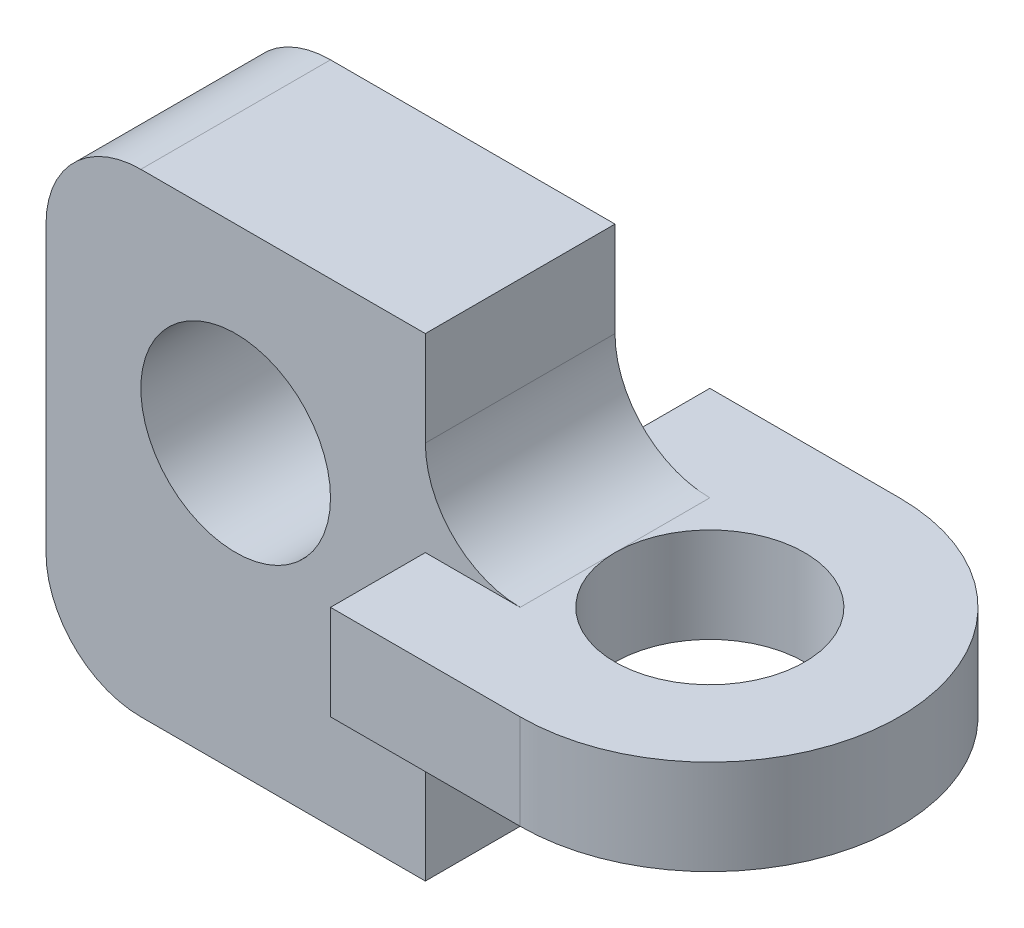
ISO-10303-21;
HEADER;
FILE_DESCRIPTION(('STEP AP214'),'2;1');
FILE_NAME('part.step','',(''),(''),'','','');
FILE_SCHEMA(('AUTOMOTIVE_DESIGN { 1 0 10303 214 1 1 1 1 }'));
ENDSEC;
DATA;
#1=APPLICATION_CONTEXT('core data for automotive mechanical design processes');
#2=APPLICATION_PROTOCOL_DEFINITION('international standard','automotive_design',2000,#1);
#3=PRODUCT_CONTEXT('',#1,'mechanical');
#4=PRODUCT('Part','Part','',(#3));
#5=PRODUCT_RELATED_PRODUCT_CATEGORY('part','',(#4));
#6=PRODUCT_DEFINITION_FORMATION('','',#4);
#7=PRODUCT_DEFINITION_CONTEXT('part definition',#1,'design');
#8=PRODUCT_DEFINITION('design','',#6,#7);
#9=PRODUCT_DEFINITION_SHAPE('','',#8);
#10=(LENGTH_UNIT() NAMED_UNIT(*) SI_UNIT(.MILLI.,.METRE.));
#11=(NAMED_UNIT(*) PLANE_ANGLE_UNIT() SI_UNIT($,.RADIAN.));
#12=(NAMED_UNIT(*) SI_UNIT($,.STERADIAN.) SOLID_ANGLE_UNIT());
#13=UNCERTAINTY_MEASURE_WITH_UNIT(LENGTH_MEASURE(1.E-05),#10,'distance_accuracy_value','');
#14=(GEOMETRIC_REPRESENTATION_CONTEXT(3) GLOBAL_UNCERTAINTY_ASSIGNED_CONTEXT((#13)) GLOBAL_UNIT_ASSIGNED_CONTEXT((#10,
#11,#12)) REPRESENTATION_CONTEXT('',''));
#15=CARTESIAN_POINT('',(0.,0.,0.));
#16=DIRECTION('',(0.,0.,1.));
#17=DIRECTION('',(1.,0.,0.));
#18=AXIS2_PLACEMENT_3D('',#15,#16,#17);
#19=CARTESIAN_POINT('',(40.,-5.,0.));
#20=DIRECTION('',(0.,-1.,0.));
#21=DIRECTION('',(0.,0.,-1.));
#22=AXIS2_PLACEMENT_3D('',#19,#20,#21);
#23=CYLINDRICAL_SURFACE('',#22,20.);
#24=DIRECTION('',(0.,-1.,0.));
#25=VECTOR('',#24,1.);
#26=CARTESIAN_POINT('',(40.,5.,20.));
#27=LINE('',#26,#25);
#28=CARTESIAN_POINT('',(40.,-5.,20.));
#29=VERTEX_POINT('',#28);
#30=CARTESIAN_POINT('',(40.,5.,20.));
#31=VERTEX_POINT('',#30);
#32=EDGE_CURVE('E178',#29,#31,#27,.F.);
#33=ORIENTED_EDGE('',*,*,#32,.F.);
#34=CARTESIAN_POINT('',(40.,-5.,0.));
#35=DIRECTION('',(0.,1.,0.));
#36=DIRECTION('',(0.,0.,1.));
#37=AXIS2_PLACEMENT_3D('',#34,#35,#36);
#38=CIRCLE('',#37,20.);
#39=CARTESIAN_POINT('',(40.,-5.,-20.));
#40=VERTEX_POINT('',#39);
#41=EDGE_CURVE('E245',#40,#29,#38,.F.);
#42=ORIENTED_EDGE('',*,*,#41,.F.);
#43=DIRECTION('',(0.,-1.,0.));
#44=VECTOR('',#43,1.);
#45=CARTESIAN_POINT('',(40.,5.,-20.));
#46=LINE('',#45,#44);
#47=CARTESIAN_POINT('',(40.,5.,-20.));
#48=VERTEX_POINT('',#47);
#49=EDGE_CURVE('E243',#48,#40,#46,.T.);
#50=ORIENTED_EDGE('',*,*,#49,.F.);
#51=CARTESIAN_POINT('',(40.,5.,0.));
#52=DIRECTION('',(0.,1.,0.));
#53=DIRECTION('',(0.,0.,1.));
#54=AXIS2_PLACEMENT_3D('',#51,#52,#53);
#55=CIRCLE('',#54,20.);
#56=EDGE_CURVE('E249',#31,#48,#55,.T.);
#57=ORIENTED_EDGE('',*,*,#56,.F.);
#58=EDGE_LOOP('',(#33,#42,#50,#57));
#59=FACE_BOUND('',#58,.T.);
#60=ADVANCED_FACE('F41',(#59),#23,.T.);
#61=CARTESIAN_POINT('',(20.,-25.,10.));
#62=DIRECTION('',(-1.,0.,0.));
#63=DIRECTION('',(0.,0.,1.));
#64=AXIS2_PLACEMENT_3D('',#61,#62,#63);
#65=PLANE('',#64);
#66=DIRECTION('',(0.,1.,0.));
#67=VECTOR('',#66,1.);
#68=CARTESIAN_POINT('',(20.,-25.,10.));
#69=LINE('',#68,#67);
#70=CARTESIAN_POINT('',(20.,15.,10.));
#71=VERTEX_POINT('',#70);
#72=CARTESIAN_POINT('',(20.,25.,10.));
#73=VERTEX_POINT('',#72);
#74=EDGE_CURVE('E203',#71,#73,#69,.T.);
#75=ORIENTED_EDGE('',*,*,#74,.F.);
#76=DIRECTION('',(0.,0.,1.));
#77=VECTOR('',#76,1.);
#78=CARTESIAN_POINT('',(20.,15.,10.));
#79=LINE('',#78,#77);
#80=CARTESIAN_POINT('',(20.,15.,-10.));
#81=VERTEX_POINT('',#80);
#82=EDGE_CURVE('E270',#71,#81,#79,.F.);
#83=ORIENTED_EDGE('',*,*,#82,.T.);
#84=DIRECTION('',(0.,1.,0.));
#85=VECTOR('',#84,1.);
#86=CARTESIAN_POINT('',(20.,-25.,-10.));
#87=LINE('',#86,#85);
#88=CARTESIAN_POINT('',(20.,25.,-10.));
#89=VERTEX_POINT('',#88);
#90=EDGE_CURVE('E188',#81,#89,#87,.T.);
#91=ORIENTED_EDGE('',*,*,#90,.T.);
#92=DIRECTION('',(0.,0.,-1.));
#93=VECTOR('',#92,1.);
#94=CARTESIAN_POINT('',(20.,25.,10.));
#95=LINE('',#94,#93);
#96=EDGE_CURVE('E240',#73,#89,#95,.T.);
#97=ORIENTED_EDGE('',*,*,#96,.F.);
#98=EDGE_LOOP('',(#75,#83,#91,#97));
#99=FACE_BOUND('',#98,.T.);
#100=ADVANCED_FACE('F282',(#99),#65,.F.);
#101=CARTESIAN_POINT('',(20.,-25.,-10.));
#102=VERTEX_POINT('',#101);
#103=CARTESIAN_POINT('',(20.,-15.,-10.));
#104=VERTEX_POINT('',#103);
#105=EDGE_CURVE('E194',#102,#104,#87,.T.);
#106=ORIENTED_EDGE('',*,*,#105,.T.);
#107=DIRECTION('',(0.,0.,1.));
#108=VECTOR('',#107,1.);
#109=CARTESIAN_POINT('',(20.,-15.,10.));
#110=LINE('',#109,#108);
#111=CARTESIAN_POINT('',(20.,-15.,10.));
#112=VERTEX_POINT('',#111);
#113=EDGE_CURVE('E250',#104,#112,#110,.T.);
#114=ORIENTED_EDGE('',*,*,#113,.T.);
#115=CARTESIAN_POINT('',(20.,-25.,10.));
#116=VERTEX_POINT('',#115);
#117=EDGE_CURVE('E198',#116,#112,#69,.T.);
#118=ORIENTED_EDGE('',*,*,#117,.F.);
#119=DIRECTION('',(0.,0.,-1.));
#120=VECTOR('',#119,1.);
#121=CARTESIAN_POINT('',(20.,-25.,10.));
#122=LINE('',#121,#120);
#123=EDGE_CURVE('E209',#116,#102,#122,.T.);
#124=ORIENTED_EDGE('',*,*,#123,.T.);
#125=EDGE_LOOP('',(#106,#114,#118,#124));
#126=FACE_BOUND('',#125,.T.);
#127=ADVANCED_FACE('F315',(#126),#65,.F.);
#128=CARTESIAN_POINT('',(20.,25.,10.));
#129=DIRECTION('',(0.,-1.,0.));
#130=DIRECTION('',(0.,0.,-1.));
#131=AXIS2_PLACEMENT_3D('',#128,#129,#130);
#132=PLANE('',#131);
#133=DIRECTION('',(-1.,0.,0.));
#134=VECTOR('',#133,1.);
#135=CARTESIAN_POINT('',(20.,25.,-10.));
#136=LINE('',#135,#134);
#137=CARTESIAN_POINT('',(-9.99999999999992,25.,-10.));
#138=VERTEX_POINT('',#137);
#139=EDGE_CURVE('E213',#89,#138,#136,.T.);
#140=ORIENTED_EDGE('',*,*,#139,.T.);
#141=DIRECTION('',(0.,0.,-1.));
#142=VECTOR('',#141,1.);
#143=CARTESIAN_POINT('',(-9.99999999999992,25.,10.));
#144=LINE('',#143,#142);
#145=CARTESIAN_POINT('',(-9.99999999999992,25.,10.));
#146=VERTEX_POINT('',#145);
#147=EDGE_CURVE('E233',#146,#138,#144,.T.);
#148=ORIENTED_EDGE('',*,*,#147,.F.);
#149=DIRECTION('',(-1.,0.,0.));
#150=VECTOR('',#149,1.);
#151=CARTESIAN_POINT('',(20.,25.,10.));
#152=LINE('',#151,#150);
#153=EDGE_CURVE('E200',#73,#146,#152,.T.);
#154=ORIENTED_EDGE('',*,*,#153,.F.);
#155=ORIENTED_EDGE('',*,*,#96,.T.);
#156=EDGE_LOOP('',(#140,#148,#154,#155));
#157=FACE_BOUND('',#156,.T.);
#158=ADVANCED_FACE('F333',(#157),#132,.F.);
#159=CARTESIAN_POINT('',(-10.,15.,10.));
#160=DIRECTION('',(0.,0.,-1.));
#161=DIRECTION('',(-1.,0.,0.));
#162=AXIS2_PLACEMENT_3D('',#159,#160,#161);
#163=CYLINDRICAL_SURFACE('',#162,10.);
#164=CARTESIAN_POINT('',(-10.,15.,-10.));
#165=DIRECTION('',(0.,0.,1.));
#166=DIRECTION('',(1.,0.,0.));
#167=AXIS2_PLACEMENT_3D('',#164,#165,#166);
#168=CIRCLE('',#167,10.);
#169=CARTESIAN_POINT('',(-20.,14.9999999999999,-10.));
#170=VERTEX_POINT('',#169);
#171=EDGE_CURVE('E214',#138,#170,#168,.T.);
#172=ORIENTED_EDGE('',*,*,#171,.T.);
#173=DIRECTION('',(0.,0.,-1.));
#174=VECTOR('',#173,1.);
#175=CARTESIAN_POINT('',(-20.,14.9999999999999,10.));
#176=LINE('',#175,#174);
#177=CARTESIAN_POINT('',(-20.,14.9999999999999,10.));
#178=VERTEX_POINT('',#177);
#179=EDGE_CURVE('E234',#178,#170,#176,.T.);
#180=ORIENTED_EDGE('',*,*,#179,.F.);
#181=CARTESIAN_POINT('',(-10.,15.,10.));
#182=DIRECTION('',(0.,0.,1.));
#183=DIRECTION('',(1.,0.,0.));
#184=AXIS2_PLACEMENT_3D('',#181,#182,#183);
#185=CIRCLE('',#184,10.);
#186=EDGE_CURVE('E201',#146,#178,#185,.T.);
#187=ORIENTED_EDGE('',*,*,#186,.F.);
#188=ORIENTED_EDGE('',*,*,#147,.T.);
#189=EDGE_LOOP('',(#172,#180,#187,#188));
#190=FACE_BOUND('',#189,.T.);
#191=ADVANCED_FACE('F335',(#190),#163,.T.);
#192=CARTESIAN_POINT('',(-20.,-14.9999999999999,10.));
#193=DIRECTION('',(1.,0.,0.));
#194=DIRECTION('',(0.,0.,-1.));
#195=AXIS2_PLACEMENT_3D('',#192,#193,#194);
#196=PLANE('',#195);
#197=DIRECTION('',(0.,-1.,0.));
#198=VECTOR('',#197,1.);
#199=CARTESIAN_POINT('',(-20.,-14.9999999999999,-10.));
#200=LINE('',#199,#198);
#201=CARTESIAN_POINT('',(-20.,-15.,-10.));
#202=VERTEX_POINT('',#201);
#203=EDGE_CURVE('E220',#170,#202,#200,.T.);
#204=ORIENTED_EDGE('',*,*,#203,.T.);
#205=DIRECTION('',(0.,0.,-1.));
#206=VECTOR('',#205,1.);
#207=CARTESIAN_POINT('',(-20.,-15.,10.));
#208=LINE('',#207,#206);
#209=CARTESIAN_POINT('',(-20.,-15.,10.));
#210=VERTEX_POINT('',#209);
#211=EDGE_CURVE('E227',#210,#202,#208,.T.);
#212=ORIENTED_EDGE('',*,*,#211,.F.);
#213=DIRECTION('',(0.,-1.,0.));
#214=VECTOR('',#213,1.);
#215=CARTESIAN_POINT('',(-20.,-14.9999999999999,10.));
#216=LINE('',#215,#214);
#217=EDGE_CURVE('E202',#178,#210,#216,.T.);
#218=ORIENTED_EDGE('',*,*,#217,.F.);
#219=ORIENTED_EDGE('',*,*,#179,.T.);
#220=EDGE_LOOP('',(#204,#212,#218,#219));
#221=FACE_BOUND('',#220,.T.);
#222=ADVANCED_FACE('F327',(#221),#196,.F.);
#223=CARTESIAN_POINT('',(-10.,-15.,10.));
#224=DIRECTION('',(0.,0.,-1.));
#225=DIRECTION('',(-1.,0.,0.));
#226=AXIS2_PLACEMENT_3D('',#223,#224,#225);
#227=CYLINDRICAL_SURFACE('',#226,10.);
#228=CARTESIAN_POINT('',(-10.,-15.,-10.));
#229=DIRECTION('',(0.,0.,1.));
#230=DIRECTION('',(-1.,0.,0.));
#231=AXIS2_PLACEMENT_3D('',#228,#229,#230);
#232=CIRCLE('',#231,10.);
#233=CARTESIAN_POINT('',(-9.99999999999993,-25.,-10.));
#234=VERTEX_POINT('',#233);
#235=EDGE_CURVE('E218',#202,#234,#232,.T.);
#236=ORIENTED_EDGE('',*,*,#235,.T.);
#237=DIRECTION('',(0.,0.,-1.));
#238=VECTOR('',#237,1.);
#239=CARTESIAN_POINT('',(-9.99999999999993,-25.,10.));
#240=LINE('',#239,#238);
#241=CARTESIAN_POINT('',(-9.99999999999993,-25.,10.));
#242=VERTEX_POINT('',#241);
#243=EDGE_CURVE('E223',#242,#234,#240,.T.);
#244=ORIENTED_EDGE('',*,*,#243,.F.);
#245=CARTESIAN_POINT('',(-10.,-15.,10.));
#246=DIRECTION('',(0.,0.,1.));
#247=DIRECTION('',(-1.,0.,0.));
#248=AXIS2_PLACEMENT_3D('',#245,#246,#247);
#249=CIRCLE('',#248,10.);
#250=EDGE_CURVE('E210',#210,#242,#249,.T.);
#251=ORIENTED_EDGE('',*,*,#250,.F.);
#252=ORIENTED_EDGE('',*,*,#211,.T.);
#253=EDGE_LOOP('',(#236,#244,#251,#252));
#254=FACE_BOUND('',#253,.T.);
#255=ADVANCED_FACE('F322',(#254),#227,.T.);
#256=CARTESIAN_POINT('',(20.,-25.,10.));
#257=DIRECTION('',(0.,1.,0.));
#258=DIRECTION('',(-1.,0.,0.));
#259=AXIS2_PLACEMENT_3D('',#256,#257,#258);
#260=PLANE('',#259);
#261=DIRECTION('',(1.,0.,0.));
#262=VECTOR('',#261,1.);
#263=CARTESIAN_POINT('',(20.,-25.,-10.));
#264=LINE('',#263,#262);
#265=EDGE_CURVE('E222',#234,#102,#264,.T.);
#266=ORIENTED_EDGE('',*,*,#265,.T.);
#267=ORIENTED_EDGE('',*,*,#123,.F.);
#268=DIRECTION('',(1.,0.,0.));
#269=VECTOR('',#268,1.);
#270=CARTESIAN_POINT('',(20.,-25.,10.));
#271=LINE('',#270,#269);
#272=EDGE_CURVE('E207',#242,#116,#271,.T.);
#273=ORIENTED_EDGE('',*,*,#272,.F.);
#274=ORIENTED_EDGE('',*,*,#243,.T.);
#275=EDGE_LOOP('',(#266,#267,#273,#274));
#276=FACE_BOUND('',#275,.T.);
#277=ADVANCED_FACE('F318',(#276),#260,.F.);
#278=CARTESIAN_POINT('',(-10.,15.,10.));
#279=DIRECTION('',(0.,0.,1.));
#280=DIRECTION('',(1.,0.,0.));
#281=AXIS2_PLACEMENT_3D('',#278,#279,#280);
#282=PLANE('',#281);
#283=CARTESIAN_POINT('',(0.,5.00000000000001,10.));
#284=DIRECTION('',(0.,0.,1.));
#285=DIRECTION('',(1.,0.,0.));
#286=AXIS2_PLACEMENT_3D('',#283,#284,#285);
#287=CIRCLE('',#286,10.);
#288=CARTESIAN_POINT('',(10.,5.00000000000001,10.));
#289=VERTEX_POINT('',#288);
#290=EDGE_CURVE('E501',#289,#289,#287,.T.);
#291=ORIENTED_EDGE('',*,*,#290,.F.);
#292=EDGE_LOOP('',(#291));
#293=FACE_BOUND('',#292,.T.);
#294=ORIENTED_EDGE('',*,*,#117,.T.);
#295=CARTESIAN_POINT('',(30.,-15.,10.));
#296=DIRECTION('',(0.,0.,1.));
#297=DIRECTION('',(1.,0.,0.));
#298=AXIS2_PLACEMENT_3D('',#295,#296,#297);
#299=CIRCLE('',#298,10.);
#300=CARTESIAN_POINT('',(30.,-5.,10.));
#301=VERTEX_POINT('',#300);
#302=EDGE_CURVE('E267',#112,#301,#299,.F.);
#303=ORIENTED_EDGE('',*,*,#302,.T.);
#304=DIRECTION('',(1.,0.,0.));
#305=VECTOR('',#304,1.);
#306=CARTESIAN_POINT('',(0.,-5.,10.));
#307=LINE('',#306,#305);
#308=CARTESIAN_POINT('',(20.,-5.,10.));
#309=VERTEX_POINT('',#308);
#310=EDGE_CURVE('E260',#309,#301,#307,.T.);
#311=ORIENTED_EDGE('',*,*,#310,.F.);
#312=CARTESIAN_POINT('',(20.,5.,10.));
#313=VERTEX_POINT('',#312);
#314=EDGE_CURVE('E199',#309,#313,#69,.T.);
#315=ORIENTED_EDGE('',*,*,#314,.T.);
#316=DIRECTION('',(-1.,0.,0.));
#317=VECTOR('',#316,1.);
#318=CARTESIAN_POINT('',(-10.,5.,10.));
#319=LINE('',#318,#317);
#320=CARTESIAN_POINT('',(30.,5.,10.));
#321=VERTEX_POINT('',#320);
#322=EDGE_CURVE('E163',#321,#313,#319,.T.);
#323=ORIENTED_EDGE('',*,*,#322,.F.);
#324=CARTESIAN_POINT('',(30.,15.,10.));
#325=DIRECTION('',(0.,0.,1.));
#326=DIRECTION('',(1.,0.,0.));
#327=AXIS2_PLACEMENT_3D('',#324,#325,#326);
#328=CIRCLE('',#327,10.);
#329=EDGE_CURVE('E49',#321,#71,#328,.F.);
#330=ORIENTED_EDGE('',*,*,#329,.T.);
#331=ORIENTED_EDGE('',*,*,#74,.T.);
#332=ORIENTED_EDGE('',*,*,#153,.T.);
#333=ORIENTED_EDGE('',*,*,#186,.T.);
#334=ORIENTED_EDGE('',*,*,#217,.T.);
#335=ORIENTED_EDGE('',*,*,#250,.T.);
#336=ORIENTED_EDGE('',*,*,#272,.T.);
#337=EDGE_LOOP('',(#294,#303,#311,#315,#323,#330,#331,#332,#333,#334,#335,#336));
#338=FACE_BOUND('',#337,.T.);
#339=ADVANCED_FACE('F277',(#293,#338),#282,.T.);
#340=CARTESIAN_POINT('',(-10.,15.,-10.));
#341=DIRECTION('',(0.,0.,1.));
#342=DIRECTION('',(1.,0.,0.));
#343=AXIS2_PLACEMENT_3D('',#340,#341,#342);
#344=PLANE('',#343);
#345=CARTESIAN_POINT('',(0.,5.00000000000001,-10.));
#346=DIRECTION('',(0.,0.,1.));
#347=DIRECTION('',(1.,0.,0.));
#348=AXIS2_PLACEMENT_3D('',#345,#346,#347);
#349=CIRCLE('',#348,10.);
#350=CARTESIAN_POINT('',(10.,5.00000000000001,-10.));
#351=VERTEX_POINT('',#350);
#352=EDGE_CURVE('E44',#351,#351,#349,.T.);
#353=ORIENTED_EDGE('',*,*,#352,.T.);
#354=EDGE_LOOP('',(#353));
#355=FACE_BOUND('',#354,.T.);
#356=ORIENTED_EDGE('',*,*,#105,.F.);
#357=ORIENTED_EDGE('',*,*,#265,.F.);
#358=ORIENTED_EDGE('',*,*,#235,.F.);
#359=ORIENTED_EDGE('',*,*,#203,.F.);
#360=ORIENTED_EDGE('',*,*,#171,.F.);
#361=ORIENTED_EDGE('',*,*,#139,.F.);
#362=ORIENTED_EDGE('',*,*,#90,.F.);
#363=CARTESIAN_POINT('',(30.,15.,-10.));
#364=DIRECTION('',(0.,0.,1.));
#365=DIRECTION('',(1.,0.,0.));
#366=AXIS2_PLACEMENT_3D('',#363,#364,#365);
#367=CIRCLE('',#366,10.);
#368=CARTESIAN_POINT('',(30.,5.,-10.));
#369=VERTEX_POINT('',#368);
#370=EDGE_CURVE('E11',#81,#369,#367,.T.);
#371=ORIENTED_EDGE('',*,*,#370,.T.);
#372=DIRECTION('',(1.,0.,0.));
#373=VECTOR('',#372,1.);
#374=CARTESIAN_POINT('',(0.,5.,-10.));
#375=LINE('',#374,#373);
#376=CARTESIAN_POINT('',(20.,5.,-10.));
#377=VERTEX_POINT('',#376);
#378=EDGE_CURVE('E257',#377,#369,#375,.T.);
#379=ORIENTED_EDGE('',*,*,#378,.F.);
#380=CARTESIAN_POINT('',(20.,-5.,-10.));
#381=VERTEX_POINT('',#380);
#382=EDGE_CURVE('E190',#381,#377,#87,.T.);
#383=ORIENTED_EDGE('',*,*,#382,.F.);
#384=DIRECTION('',(-1.,0.,0.));
#385=VECTOR('',#384,1.);
#386=CARTESIAN_POINT('',(-10.,-5.,-10.));
#387=LINE('',#386,#385);
#388=CARTESIAN_POINT('',(30.,-5.,-10.));
#389=VERTEX_POINT('',#388);
#390=EDGE_CURVE('E253',#389,#381,#387,.T.);
#391=ORIENTED_EDGE('',*,*,#390,.F.);
#392=CARTESIAN_POINT('',(30.,-15.,-10.));
#393=DIRECTION('',(0.,0.,1.));
#394=DIRECTION('',(1.,0.,0.));
#395=AXIS2_PLACEMENT_3D('',#392,#393,#394);
#396=CIRCLE('',#395,10.);
#397=EDGE_CURVE('E271',#389,#104,#396,.T.);
#398=ORIENTED_EDGE('',*,*,#397,.T.);
#399=EDGE_LOOP('',(#356,#357,#358,#359,#360,#361,#362,#371,#379,#383,#391,#398));
#400=FACE_BOUND('',#399,.T.);
#401=ADVANCED_FACE('F288',(#355,#400),#344,.F.);
#402=CARTESIAN_POINT('',(20.,5.,20.));
#403=DIRECTION('',(1.,0.,0.));
#404=DIRECTION('',(0.,0.,-1.));
#405=AXIS2_PLACEMENT_3D('',#402,#403,#404);
#406=PLANE('',#405);
#407=DIRECTION('',(0.,0.,1.));
#408=VECTOR('',#407,1.);
#409=CARTESIAN_POINT('',(20.,-5.,20.));
#410=LINE('',#409,#408);
#411=CARTESIAN_POINT('',(20.,-5.,-20.));
#412=VERTEX_POINT('',#411);
#413=EDGE_CURVE('E304',#412,#381,#410,.T.);
#414=ORIENTED_EDGE('',*,*,#413,.T.);
#415=ORIENTED_EDGE('',*,*,#382,.T.);
#416=DIRECTION('',(0.,0.,1.));
#417=VECTOR('',#416,1.);
#418=CARTESIAN_POINT('',(20.,5.,20.));
#419=LINE('',#418,#417);
#420=CARTESIAN_POINT('',(20.,5.,-20.));
#421=VERTEX_POINT('',#420);
#422=EDGE_CURVE('E166',#421,#377,#419,.T.);
#423=ORIENTED_EDGE('',*,*,#422,.F.);
#424=DIRECTION('',(0.,-1.,0.));
#425=VECTOR('',#424,1.);
#426=CARTESIAN_POINT('',(20.,5.,-20.));
#427=LINE('',#426,#425);
#428=EDGE_CURVE('E189',#421,#412,#427,.T.);
#429=ORIENTED_EDGE('',*,*,#428,.T.);
#430=EDGE_LOOP('',(#414,#415,#423,#429));
#431=FACE_BOUND('',#430,.T.);
#432=ADVANCED_FACE('F300',(#431),#406,.F.);
#433=ORIENTED_EDGE('',*,*,#314,.F.);
#434=CARTESIAN_POINT('',(20.,-5.,20.));
#435=VERTEX_POINT('',#434);
#436=EDGE_CURVE('E184',#309,#435,#410,.T.);
#437=ORIENTED_EDGE('',*,*,#436,.T.);
#438=DIRECTION('',(0.,-1.,0.));
#439=VECTOR('',#438,1.);
#440=CARTESIAN_POINT('',(20.,5.,20.));
#441=LINE('',#440,#439);
#442=CARTESIAN_POINT('',(20.,5.,20.));
#443=VERTEX_POINT('',#442);
#444=EDGE_CURVE('E176',#443,#435,#441,.T.);
#445=ORIENTED_EDGE('',*,*,#444,.F.);
#446=EDGE_CURVE('E158',#313,#443,#419,.T.);
#447=ORIENTED_EDGE('',*,*,#446,.F.);
#448=EDGE_LOOP('',(#433,#437,#445,#447));
#449=FACE_BOUND('',#448,.T.);
#450=ADVANCED_FACE('F185',(#449),#406,.F.);
#451=CARTESIAN_POINT('',(60.,5.,20.));
#452=DIRECTION('',(0.,0.,-1.));
#453=DIRECTION('',(-1.,0.,0.));
#454=AXIS2_PLACEMENT_3D('',#451,#452,#453);
#455=PLANE('',#454);
#456=DIRECTION('',(1.,0.,0.));
#457=VECTOR('',#456,1.);
#458=CARTESIAN_POINT('',(60.,-5.,20.));
#459=LINE('',#458,#457);
#460=EDGE_CURVE('E514',#435,#29,#459,.T.);
#461=ORIENTED_EDGE('',*,*,#460,.T.);
#462=ORIENTED_EDGE('',*,*,#32,.T.);
#463=DIRECTION('',(1.,0.,0.));
#464=VECTOR('',#463,1.);
#465=CARTESIAN_POINT('',(60.,5.,20.));
#466=LINE('',#465,#464);
#467=EDGE_CURVE('E165',#443,#31,#466,.T.);
#468=ORIENTED_EDGE('',*,*,#467,.F.);
#469=ORIENTED_EDGE('',*,*,#444,.T.);
#470=EDGE_LOOP('',(#461,#462,#468,#469));
#471=FACE_BOUND('',#470,.T.);
#472=ADVANCED_FACE('F179',(#471),#455,.F.);
#473=CARTESIAN_POINT('',(60.,5.,-20.));
#474=DIRECTION('',(0.,0.,1.));
#475=DIRECTION('',(1.,0.,0.));
#476=AXIS2_PLACEMENT_3D('',#473,#474,#475);
#477=PLANE('',#476);
#478=DIRECTION('',(-1.,0.,0.));
#479=VECTOR('',#478,1.);
#480=CARTESIAN_POINT('',(60.,5.,-20.));
#481=LINE('',#480,#479);
#482=EDGE_CURVE('E177',#48,#421,#481,.T.);
#483=ORIENTED_EDGE('',*,*,#482,.F.);
#484=ORIENTED_EDGE('',*,*,#49,.T.);
#485=DIRECTION('',(-1.,0.,0.));
#486=VECTOR('',#485,1.);
#487=CARTESIAN_POINT('',(60.,-5.,-20.));
#488=LINE('',#487,#486);
#489=EDGE_CURVE('E168',#40,#412,#488,.T.);
#490=ORIENTED_EDGE('',*,*,#489,.T.);
#491=ORIENTED_EDGE('',*,*,#428,.F.);
#492=EDGE_LOOP('',(#483,#484,#490,#491));
#493=FACE_BOUND('',#492,.T.);
#494=ADVANCED_FACE('F368',(#493),#477,.F.);
#495=CARTESIAN_POINT('',(0.,5.,0.));
#496=DIRECTION('',(0.,1.,0.));
#497=DIRECTION('',(0.,0.,1.));
#498=AXIS2_PLACEMENT_3D('',#495,#496,#497);
#499=PLANE('',#498);
#500=DIRECTION('',(0.,0.,1.));
#501=VECTOR('',#500,1.);
#502=CARTESIAN_POINT('',(30.,5.,0.));
#503=LINE('',#502,#501);
#504=CARTESIAN_POINT('',(30.,5.,0.));
#505=VERTEX_POINT('',#504);
#506=EDGE_CURVE('E262',#369,#505,#503,.T.);
#507=ORIENTED_EDGE('',*,*,#506,.T.);
#508=CARTESIAN_POINT('',(40.,5.,0.));
#509=DIRECTION('',(0.,1.,0.));
#510=DIRECTION('',(0.,0.,1.));
#511=AXIS2_PLACEMENT_3D('',#508,#509,#510);
#512=CIRCLE('',#511,10.);
#513=EDGE_CURVE('E58',#505,#505,#512,.T.);
#514=ORIENTED_EDGE('',*,*,#513,.F.);
#515=EDGE_CURVE('E263',#505,#321,#503,.T.);
#516=ORIENTED_EDGE('',*,*,#515,.T.);
#517=ORIENTED_EDGE('',*,*,#322,.T.);
#518=ORIENTED_EDGE('',*,*,#446,.T.);
#519=ORIENTED_EDGE('',*,*,#467,.T.);
#520=ORIENTED_EDGE('',*,*,#56,.T.);
#521=ORIENTED_EDGE('',*,*,#482,.T.);
#522=ORIENTED_EDGE('',*,*,#422,.T.);
#523=ORIENTED_EDGE('',*,*,#378,.T.);
#524=EDGE_LOOP('',(#507,#514,#516,#517,#518,#519,#520,#521,#522,#523));
#525=FACE_BOUND('',#524,.T.);
#526=ADVANCED_FACE('F161',(#525),#499,.T.);
#527=CARTESIAN_POINT('',(0.,-5.,0.));
#528=DIRECTION('',(0.,1.,0.));
#529=DIRECTION('',(0.,0.,1.));
#530=AXIS2_PLACEMENT_3D('',#527,#528,#529);
#531=PLANE('',#530);
#532=DIRECTION('',(0.,0.,1.));
#533=VECTOR('',#532,1.);
#534=CARTESIAN_POINT('',(30.,-5.,-10.));
#535=LINE('',#534,#533);
#536=CARTESIAN_POINT('',(30.,-5.,0.));
#537=VERTEX_POINT('',#536);
#538=EDGE_CURVE('E255',#301,#537,#535,.F.);
#539=ORIENTED_EDGE('',*,*,#538,.T.);
#540=CARTESIAN_POINT('',(40.,-5.,0.));
#541=DIRECTION('',(0.,1.,0.));
#542=DIRECTION('',(0.,0.,1.));
#543=AXIS2_PLACEMENT_3D('',#540,#541,#542);
#544=CIRCLE('',#543,10.);
#545=EDGE_CURVE('E54',#537,#537,#544,.T.);
#546=ORIENTED_EDGE('',*,*,#545,.T.);
#547=EDGE_CURVE('E251',#537,#389,#535,.F.);
#548=ORIENTED_EDGE('',*,*,#547,.T.);
#549=ORIENTED_EDGE('',*,*,#390,.T.);
#550=ORIENTED_EDGE('',*,*,#413,.F.);
#551=ORIENTED_EDGE('',*,*,#489,.F.);
#552=ORIENTED_EDGE('',*,*,#41,.T.);
#553=ORIENTED_EDGE('',*,*,#460,.F.);
#554=ORIENTED_EDGE('',*,*,#436,.F.);
#555=ORIENTED_EDGE('',*,*,#310,.T.);
#556=EDGE_LOOP('',(#539,#546,#548,#549,#550,#551,#552,#553,#554,#555));
#557=FACE_BOUND('',#556,.T.);
#558=ADVANCED_FACE('F359',(#557),#531,.F.);
#559=CARTESIAN_POINT('',(30.,-15.,10.));
#560=DIRECTION('',(0.,0.,-1.));
#561=DIRECTION('',(-1.,0.,0.));
#562=AXIS2_PLACEMENT_3D('',#559,#560,#561);
#563=CYLINDRICAL_SURFACE('',#562,10.);
#564=ORIENTED_EDGE('',*,*,#397,.F.);
#565=ORIENTED_EDGE('',*,*,#547,.F.);
#566=ORIENTED_EDGE('',*,*,#538,.F.);
#567=ORIENTED_EDGE('',*,*,#302,.F.);
#568=ORIENTED_EDGE('',*,*,#113,.F.);
#569=EDGE_LOOP('',(#564,#565,#566,#567,#568));
#570=FACE_BOUND('',#569,.T.);
#571=ADVANCED_FACE('F306',(#570),#563,.F.);
#572=CARTESIAN_POINT('',(30.,15.,0.));
#573=DIRECTION('',(0.,0.,1.));
#574=DIRECTION('',(1.,0.,0.));
#575=AXIS2_PLACEMENT_3D('',#572,#573,#574);
#576=CYLINDRICAL_SURFACE('',#575,10.);
#577=ORIENTED_EDGE('',*,*,#370,.F.);
#578=ORIENTED_EDGE('',*,*,#82,.F.);
#579=ORIENTED_EDGE('',*,*,#329,.F.);
#580=ORIENTED_EDGE('',*,*,#515,.F.);
#581=ORIENTED_EDGE('',*,*,#506,.F.);
#582=EDGE_LOOP('',(#577,#578,#579,#580,#581));
#583=FACE_BOUND('',#582,.T.);
#584=ADVANCED_FACE('F43',(#583),#576,.F.);
#585=CARTESIAN_POINT('',(0.,5.00000000000001,-20.));
#586=DIRECTION('',(0.,0.,1.));
#587=DIRECTION('',(1.,0.,0.));
#588=AXIS2_PLACEMENT_3D('',#585,#586,#587);
#589=CYLINDRICAL_SURFACE('',#588,10.);
#590=ORIENTED_EDGE('',*,*,#290,.T.);
#591=EDGE_LOOP('',(#590));
#592=FACE_BOUND('',#591,.T.);
#593=ORIENTED_EDGE('',*,*,#352,.F.);
#594=EDGE_LOOP('',(#593));
#595=FACE_BOUND('',#594,.T.);
#596=ADVANCED_FACE('F363',(#592,#595),#589,.F.);
#597=CARTESIAN_POINT('',(40.,-25.,0.));
#598=DIRECTION('',(0.,1.,0.));
#599=DIRECTION('',(0.,0.,1.));
#600=AXIS2_PLACEMENT_3D('',#597,#598,#599);
#601=CYLINDRICAL_SURFACE('',#600,10.);
#602=ORIENTED_EDGE('',*,*,#513,.T.);
#603=EDGE_LOOP('',(#602));
#604=FACE_BOUND('',#603,.T.);
#605=ORIENTED_EDGE('',*,*,#545,.F.);
#606=EDGE_LOOP('',(#605));
#607=FACE_BOUND('',#606,.T.);
#608=ADVANCED_FACE('F456',(#604,#607),#601,.F.);
#609=CLOSED_SHELL('',(#60,#100,#127,#158,#191,#222,#255,#277,#339,#401,#432,#450,#472,#494,#526,
#558,#571,#584,#596,#608));
#610=MANIFOLD_SOLID_BREP('B2',#609);
#611=ADVANCED_BREP_SHAPE_REPRESENTATION('',(#18,#610),#14);
#612=SHAPE_DEFINITION_REPRESENTATION(#9,#611);
ENDSEC;
END-ISO-10303-21;
